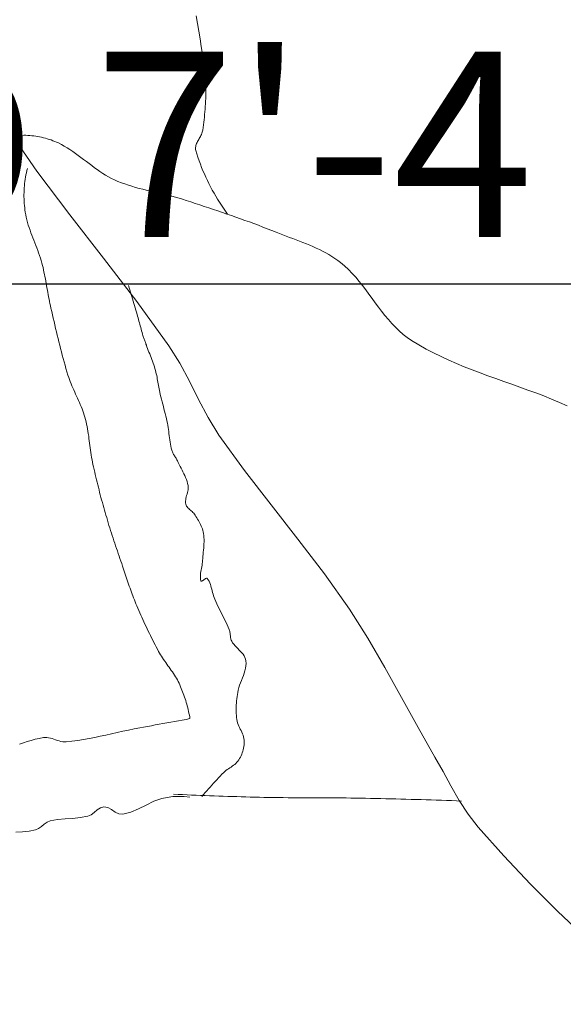
# Model space of a CAD drawing. Units: inches. Extents: x 2656 to 9931, y 1941 to 3068.
# Tile 17 of 46: x 2896 to 2914, y 2466 to 2498. Entities that reach past the tile are written whole.
import ezdxf

# ---------------------------------------------------------------- set-up
doc = ezdxf.new("R2010")
doc.units = ezdxf.units.IN
doc.layers.add('A-ANNO-DIMS', color=2, linetype='Continuous', lineweight=18)
doc.layers.add('A-FURN', color=8, linetype='Continuous', lineweight=13)
doc.styles.get("Standard").update_dxf_attribs({"font": 'arial.ttf'})
doc.dimstyles.new('ISO-25', dxfattribs={"dimtxt": 6, "dimasz": 2.5, "dimexe": 1.25, "dimexo": 0.625, "dimtad": 1, "dimdec": 0, "dimlunit": 3, "dimtxsty": 'Standard', "dimcen": 2.5, "dimadec": 0, "dimazin": 0, "dimtfac": 1, "dimtdec": 0, "dimtmove": 0, "dimatfit": 3, "dimfxl": 1, "dimarcsym": 0})

# ---------------------------------------------------------------- blocks, each defined once
blk = doc.blocks.new('BED-DOUBLE')
for p, q in [((24.852, 30.888), (24.895, 30.639)), ((24.895, 30.639), (24.937, 30.391)), ((24.937, 30.391), (24.978, 30.142)), ((24.978, 30.142), (25.017, 29.893)), ((25.017, 29.893), (25.054, 29.644)), ((25.054, 29.644), (25.087, 29.395)), ((25.087, 29.395), (25.118, 29.145)), ((25.118, 29.145), (25.146, 28.894)), ((25.146, 28.894), (25.153, 28.81)), ((25.153, 28.81), (25.159, 28.725)), ((25.159, 28.725), (25.164, 28.64)), ((25.164, 28.64), (25.166, 28.554)), ((25.166, 28.554), (25.168, 28.469)), ((25.168, 28.384), (25.166, 28.299)), ((25.168, 28.469), (25.168, 28.384)), ((25.155, 28.042), (25.149, 27.957)), ((25.16, 28.128), (25.155, 28.042)), ((25.163, 28.213), (25.16, 28.128)), ((25.166, 28.299), (25.163, 28.213)), ((25.127, 27.701), (25.118, 27.616)), ((25.135, 27.787), (25.127, 27.701)), ((25.142, 27.872), (25.135, 27.787)), ((25.149, 27.957), (25.142, 27.872)), ((25.098, 27.446), (25.088, 27.361)), ((25.108, 27.531), (25.098, 27.446)), ((25.118, 27.616), (25.108, 27.531)), ((18.699, 27.32), (19.702, 25.863)), ((25.04, 27.09), (25.026, 27.056)), ((25.052, 27.124), (25.04, 27.09)), ((25.061, 27.158), (25.052, 27.124)), ((25.067, 27.192), (25.061, 27.158)), ((25.078, 27.276), (25.067, 27.192)), ((25.088, 27.361), (25.078, 27.276)), ((19.217, 27.024), (19.153, 27.022)), ((19.28, 27.025), (19.217, 27.024)), ((19.344, 27.025), (19.28, 27.025)), ((19.408, 27.022), (19.344, 27.025)), ((19.472, 27.018), (19.408, 27.022)), ((19.535, 27.013), (19.472, 27.018)), ((19.599, 27.006), (19.535, 27.013)), ((19.663, 26.997), (19.599, 27.006)), ((19.726, 26.987), (19.663, 26.997)), ((19.789, 26.975), (19.726, 26.987)), ((19.852, 26.962), (19.789, 26.975)), ((19.915, 26.947), (19.852, 26.962)), ((19.977, 26.931), (19.915, 26.947)), ((20.039, 26.914), (19.977, 26.931)), ((20.1, 26.895), (20.039, 26.914)), ((20.16, 26.874), (20.1, 26.895)), ((20.22, 26.852), (20.16, 26.874)), ((20.28, 26.829), (20.22, 26.852)), ((20.338, 26.804), (20.28, 26.829)), ((20.396, 26.778), (20.338, 26.804)), ((20.493, 26.729), (20.396, 26.778)), ((24.869, 26.763), (24.856, 26.73)), ((24.884, 26.795), (24.869, 26.763)), ((24.901, 26.827), (24.884, 26.795)), ((24.919, 26.86), (24.901, 26.827)), ((24.937, 26.892), (24.919, 26.86)), ((24.956, 26.925), (24.937, 26.892)), ((24.975, 26.958), (24.956, 26.925)), ((24.993, 26.99), (24.975, 26.958)), ((25.01, 27.023), (24.993, 26.99)), ((25.026, 27.056), (25.01, 27.023)), ((20.588, 26.677), (20.493, 26.729)), ((20.681, 26.622), (20.588, 26.677)), ((20.773, 26.564), (20.681, 26.622)), ((20.863, 26.503), (20.773, 26.564)), ((20.952, 26.44), (20.863, 26.503)), ((21.04, 26.376), (20.952, 26.44)), ((24.833, 26.633), (24.832, 26.6)), ((24.832, 26.6), (24.835, 26.567)), ((24.838, 26.665), (24.833, 26.633)), ((24.835, 26.567), (24.842, 26.534)), ((24.845, 26.698), (24.838, 26.665)), ((24.842, 26.534), (24.876, 26.424)), ((24.856, 26.73), (24.845, 26.698)), ((24.876, 26.424), (24.912, 26.314)), ((21.128, 26.31), (21.04, 26.376)), ((21.215, 26.244), (21.128, 26.31)), ((21.302, 26.177), (21.215, 26.244)), ((21.389, 26.11), (21.302, 26.177)), ((21.476, 26.044), (21.389, 26.11)), ((24.912, 26.314), (24.949, 26.205)), ((24.949, 26.205), (24.989, 26.097)), ((19.362, 25.817), (19.348, 25.747)), ((19.377, 25.886), (19.362, 25.817)), ((19.394, 25.954), (19.377, 25.886)), ((19.702, 25.863), (20.765, 24.449)), ((21.563, 25.979), (21.476, 26.044)), ((21.652, 25.915), (21.563, 25.979)), ((21.741, 25.853), (21.652, 25.915)), ((21.832, 25.793), (21.741, 25.853)), ((21.924, 25.736), (21.832, 25.793)), ((24.989, 26.097), (25.031, 25.989)), ((25.031, 25.989), (25.074, 25.882)), ((25.074, 25.882), (25.12, 25.776)), ((19.314, 25.537), (19.306, 25.466)), ((19.324, 25.607), (19.314, 25.537)), ((19.335, 25.677), (19.324, 25.607)), ((19.348, 25.747), (19.335, 25.677)), ((22.018, 25.682), (21.924, 25.736)), ((22.114, 25.632), (22.018, 25.682)), ((22.211, 25.585), (22.114, 25.632)), ((22.322, 25.537), (22.211, 25.585)), ((22.434, 25.493), (22.322, 25.537)), ((22.547, 25.452), (22.434, 25.493)), ((25.12, 25.776), (25.167, 25.671)), ((25.167, 25.671), (25.216, 25.566)), ((25.216, 25.566), (25.267, 25.462)), ((19.286, 25.181), (19.285, 25.11)), ((19.289, 25.253), (19.286, 25.181)), ((19.293, 25.324), (19.289, 25.253)), ((19.299, 25.395), (19.293, 25.324)), ((19.306, 25.466), (19.299, 25.395)), ((22.661, 25.413), (22.547, 25.452)), ((22.775, 25.377), (22.661, 25.413)), ((22.891, 25.343), (22.775, 25.377)), ((23.007, 25.311), (22.891, 25.343)), ((23.124, 25.28), (23.007, 25.311)), ((23.241, 25.25), (23.124, 25.28)), ((23.359, 25.222), (23.241, 25.25)), ((23.476, 25.194), (23.359, 25.222)), ((23.594, 25.166), (23.476, 25.194)), ((23.712, 25.138), (23.594, 25.166)), ((25.267, 25.462), (25.32, 25.359)), ((25.32, 25.359), (25.374, 25.257)), ((25.374, 25.257), (25.431, 25.156)), ((25.431, 25.156), (25.489, 25.056)), ((19.285, 25.11), (19.285, 25.039)), ((19.285, 25.039), (19.287, 24.968)), ((19.287, 24.968), (19.289, 24.897)), ((19.289, 24.897), (19.294, 24.826)), ((23.83, 25.11), (23.712, 25.138)), ((23.948, 25.082), (23.83, 25.11)), ((24.065, 25.053), (23.948, 25.082)), ((24.182, 25.022), (24.065, 25.053)), ((24.299, 24.99), (24.182, 25.022)), ((24.414, 24.956), (24.299, 24.99)), ((24.53, 24.92), (24.414, 24.956)), ((24.676, 24.872), (24.53, 24.92)), ((24.823, 24.824), (24.676, 24.872)), ((25.489, 25.056), (25.548, 24.957)), ((25.548, 24.957), (25.61, 24.859)), ((25.61, 24.859), (25.673, 24.762)), ((19.294, 24.826), (19.3, 24.755)), ((19.3, 24.755), (19.307, 24.684)), ((19.307, 24.684), (19.315, 24.614)), ((19.315, 24.614), (19.325, 24.544)), ((19.325, 24.544), (19.34, 24.459)), ((24.97, 24.776), (24.823, 24.824)), ((25.117, 24.728), (24.97, 24.776)), ((25.263, 24.679), (25.117, 24.728)), ((25.41, 24.63), (25.263, 24.679)), ((25.556, 24.581), (25.41, 24.63)), ((25.702, 24.531), (25.556, 24.581)), ((25.673, 24.762), (25.737, 24.667)), ((25.848, 24.481), (25.702, 24.531)), ((25.737, 24.667), (25.804, 24.573)), ((25.804, 24.573), (25.871, 24.48)), ((19.34, 24.459), (19.358, 24.374)), ((19.358, 24.374), (19.378, 24.29)), ((19.378, 24.29), (19.401, 24.206)), ((19.401, 24.206), (19.425, 24.123)), ((20.765, 24.449), (21.855, 23.052)), ((25.994, 24.431), (25.848, 24.481)), ((26.14, 24.38), (25.994, 24.431)), ((26.285, 24.328), (26.14, 24.38)), ((26.431, 24.276), (26.285, 24.328)), ((26.576, 24.223), (26.431, 24.276)), ((26.72, 24.169), (26.576, 24.223)), ((19.425, 24.123), (19.452, 24.04)), ((19.452, 24.04), (19.48, 23.958)), ((19.48, 23.958), (19.509, 23.876)), ((19.509, 23.876), (19.54, 23.794)), ((26.865, 24.115), (26.72, 24.169)), ((27.009, 24.06), (26.865, 24.115)), ((27.153, 24.005), (27.009, 24.06)), ((27.297, 23.949), (27.153, 24.005)), ((27.44, 23.891), (27.297, 23.949)), ((27.548, 23.849), (27.44, 23.891)), ((19.54, 23.794), (19.571, 23.713)), ((19.571, 23.713), (19.603, 23.631)), ((19.603, 23.631), (19.635, 23.55)), ((27.656, 23.807), (27.548, 23.849)), ((27.764, 23.766), (27.656, 23.807)), ((27.873, 23.726), (27.764, 23.766)), ((27.982, 23.685), (27.873, 23.726)), ((28.092, 23.644), (27.982, 23.685)), ((28.201, 23.603), (28.092, 23.644)), ((28.309, 23.561), (28.201, 23.603)), ((28.418, 23.518), (28.309, 23.561)), ((19.635, 23.55), (19.666, 23.468)), ((19.666, 23.468), (19.698, 23.387)), ((19.698, 23.387), (19.729, 23.305)), ((19.729, 23.305), (19.758, 23.223)), ((28.525, 23.474), (28.418, 23.518)), ((28.632, 23.428), (28.525, 23.474)), ((28.738, 23.381), (28.632, 23.428)), ((28.842, 23.332), (28.738, 23.381)), ((28.945, 23.28), (28.842, 23.332)), ((29.047, 23.227), (28.945, 23.28)), ((19.758, 23.223), (19.787, 23.141)), ((19.787, 23.141), (19.814, 23.058)), ((19.814, 23.058), (19.84, 22.975)), ((19.84, 22.975), (19.864, 22.891)), ((21.855, 23.052), (22.936, 21.65)), ((29.147, 23.17), (29.047, 23.227)), ((29.245, 23.11), (29.147, 23.17)), ((29.341, 23.048), (29.245, 23.11)), ((29.434, 22.981), (29.341, 23.048)), ((29.526, 22.911), (29.434, 22.981)), ((19.864, 22.891), (19.882, 22.819)), ((19.882, 22.819), (19.9, 22.747)), ((19.9, 22.747), (19.917, 22.675)), ((19.917, 22.675), (19.932, 22.603)), ((19.932, 22.603), (19.947, 22.53)), ((29.656, 22.802), (29.526, 22.911)), ((29.78, 22.685), (29.656, 22.802)), ((29.898, 22.563), (29.78, 22.685)), ((19.947, 22.53), (19.962, 22.458)), ((19.962, 22.458), (19.976, 22.385)), ((19.976, 22.385), (19.99, 22.312)), ((19.99, 22.312), (20.003, 22.239)), ((30.013, 22.435), (29.898, 22.563)), ((30.123, 22.304), (30.013, 22.435)), ((30.231, 22.169), (30.123, 22.304)), ((20.003, 22.239), (20.016, 22.166)), ((20.016, 22.166), (20.029, 22.093)), ((20.029, 22.093), (20.042, 22.02)), ((20.042, 22.02), (20.055, 21.947)), ((22.664, 22.169), (22.686, 22.097)), ((22.686, 22.097), (22.708, 22.025)), ((22.708, 22.025), (22.73, 21.953)), ((30.336, 22.032), (30.231, 22.169)), ((30.44, 21.893), (30.336, 22.032)), ((20.055, 21.947), (20.068, 21.874)), ((20.068, 21.874), (20.082, 21.801)), ((20.082, 21.801), (20.095, 21.728)), ((20.095, 21.728), (20.11, 21.655)), ((20.11, 21.655), (20.125, 21.583)), ((22.73, 21.953), (22.752, 21.881)), ((22.752, 21.881), (22.774, 21.809)), ((22.774, 21.809), (22.796, 21.737)), ((22.796, 21.737), (22.817, 21.665)), ((22.817, 21.665), (22.839, 21.592)), ((22.936, 21.65), (23.974, 20.217)), ((30.543, 21.753), (30.44, 21.893)), ((30.646, 21.613), (30.543, 21.753)), ((20.125, 21.583), (20.14, 21.51)), ((20.14, 21.51), (20.157, 21.438)), ((20.157, 21.438), (20.182, 21.329)), ((20.182, 21.329), (20.207, 21.22)), ((22.839, 21.592), (22.86, 21.52)), ((22.86, 21.52), (22.881, 21.448)), ((22.881, 21.448), (22.902, 21.376)), ((22.902, 21.376), (22.923, 21.303)), ((30.749, 21.474), (30.646, 21.613)), ((30.853, 21.336), (30.749, 21.474)), ((30.96, 21.201), (30.853, 21.336)), ((20.207, 21.22), (20.232, 21.111)), ((20.232, 21.111), (20.258, 21.002)), ((22.923, 21.303), (22.944, 21.231)), ((22.944, 21.231), (22.959, 21.179)), ((22.959, 21.179), (22.974, 21.126)), ((22.974, 21.126), (22.988, 21.074)), ((22.988, 21.074), (23.003, 21.021)), ((23.003, 21.021), (23.017, 20.968)), ((31.069, 21.069), (30.96, 21.201)), ((31.181, 20.941), (31.069, 21.069)), ((20.258, 21.002), (20.283, 20.893)), ((20.283, 20.893), (20.308, 20.784)), ((20.308, 20.784), (20.334, 20.675)), ((23.017, 20.968), (23.03, 20.916)), ((23.03, 20.916), (23.044, 20.863)), ((23.044, 20.863), (23.059, 20.81)), ((23.059, 20.81), (23.073, 20.758)), ((23.073, 20.758), (23.087, 20.705)), ((23.087, 20.705), (23.102, 20.653)), ((31.298, 20.818), (31.181, 20.941)), ((31.419, 20.7), (31.298, 20.818)), ((31.546, 20.59), (31.419, 20.7)), ((20.334, 20.675), (20.36, 20.566)), ((20.36, 20.566), (20.386, 20.457)), ((20.386, 20.457), (20.412, 20.349)), ((23.102, 20.653), (23.117, 20.601)), ((23.117, 20.601), (23.133, 20.548)), ((23.133, 20.548), (23.142, 20.521)), ((23.142, 20.521), (23.151, 20.493)), ((23.151, 20.493), (23.16, 20.465)), ((23.16, 20.465), (23.17, 20.438)), ((23.17, 20.438), (23.18, 20.41)), ((23.18, 20.41), (23.19, 20.383)), ((23.19, 20.383), (23.2, 20.355)), ((31.68, 20.486), (31.546, 20.59)), ((31.82, 20.391), (31.68, 20.486)), ((32.053, 20.249), (31.82, 20.391)), ((20.412, 20.349), (20.439, 20.24)), ((20.439, 20.24), (20.467, 20.131)), ((20.467, 20.131), (20.494, 20.023)), ((23.2, 20.355), (23.211, 20.328)), ((23.211, 20.328), (23.221, 20.301)), ((23.221, 20.301), (23.231, 20.273)), ((23.231, 20.273), (23.242, 20.246)), ((23.242, 20.246), (23.252, 20.218)), ((23.252, 20.218), (23.262, 20.191)), ((23.262, 20.191), (23.283, 20.132)), ((23.283, 20.132), (23.305, 20.073)), ((23.305, 20.073), (23.328, 20.015)), ((23.974, 20.217), (24.323, 19.656)), ((32.29, 20.116), (32.053, 20.249)), ((32.531, 19.99), (32.29, 20.116)), ((20.494, 20.023), (20.523, 19.915)), ((20.523, 19.915), (20.552, 19.807)), ((20.552, 19.807), (20.581, 19.699)), ((23.328, 20.015), (23.35, 19.956)), ((23.35, 19.956), (23.373, 19.898)), ((23.373, 19.898), (23.396, 19.839)), ((23.396, 19.839), (23.418, 19.781)), ((23.418, 19.781), (23.44, 19.722)), ((32.775, 19.87), (32.531, 19.99)), ((33.022, 19.757), (32.775, 19.87)), ((33.272, 19.649), (33.022, 19.757)), ((20.581, 19.699), (20.612, 19.591)), ((20.612, 19.591), (20.643, 19.484)), ((20.643, 19.484), (20.675, 19.377)), ((23.44, 19.722), (23.461, 19.663)), ((23.461, 19.663), (23.482, 19.604)), ((23.482, 19.604), (23.502, 19.544)), ((23.502, 19.544), (23.521, 19.485)), ((23.521, 19.485), (23.538, 19.425)), ((23.538, 19.425), (23.552, 19.372)), ((24.323, 19.656), (24.634, 19.073)), ((33.525, 19.545), (33.272, 19.649)), ((33.779, 19.445), (33.525, 19.545)), ((34.035, 19.348), (33.779, 19.445)), ((20.675, 19.377), (20.708, 19.27)), ((20.708, 19.27), (20.73, 19.2)), ((20.73, 19.2), (20.755, 19.131)), ((20.755, 19.131), (20.781, 19.062)), ((23.552, 19.372), (23.565, 19.318)), ((23.565, 19.318), (23.577, 19.265)), ((23.577, 19.265), (23.587, 19.211)), ((23.587, 19.211), (23.597, 19.157)), ((23.597, 19.157), (23.607, 19.102)), ((23.607, 19.102), (23.616, 19.048)), ((34.292, 19.254), (34.035, 19.348)), ((34.55, 19.161), (34.292, 19.254)), ((34.809, 19.069), (34.55, 19.161)), ((20.781, 19.062), (20.808, 18.994)), ((20.808, 18.994), (20.836, 18.926)), ((20.836, 18.926), (20.865, 18.859)), ((20.865, 18.859), (20.895, 18.792)), ((20.895, 18.792), (20.925, 18.725)), ((23.616, 19.048), (23.625, 18.994)), ((23.625, 18.994), (23.634, 18.94)), ((23.634, 18.94), (23.643, 18.885)), ((23.643, 18.885), (23.653, 18.831)), ((23.653, 18.831), (23.664, 18.777)), ((24.634, 19.073), (24.932, 18.481)), ((35.068, 18.977), (34.809, 19.069)), ((35.326, 18.885), (35.068, 18.977)), ((35.584, 18.791), (35.326, 18.885)), ((35.841, 18.696), (35.584, 18.791)), ((20.925, 18.725), (20.956, 18.658)), ((20.956, 18.658), (20.987, 18.591)), ((20.987, 18.591), (21.017, 18.524)), ((21.017, 18.524), (21.048, 18.457)), ((23.664, 18.777), (23.675, 18.724)), ((23.675, 18.724), (23.693, 18.646)), ((23.693, 18.646), (23.712, 18.568)), ((23.712, 18.568), (23.732, 18.491)), ((23.732, 18.491), (23.751, 18.414)), ((24.932, 18.481), (25.243, 17.897)), ((36.097, 18.598), (35.841, 18.696)), ((36.351, 18.496), (36.097, 18.598)), ((36.603, 18.391), (36.351, 18.496)), ((21.048, 18.457), (21.078, 18.39)), ((21.078, 18.39), (21.107, 18.322)), ((21.107, 18.322), (21.135, 18.255)), ((21.135, 18.255), (21.162, 18.186)), ((21.162, 18.186), (21.188, 18.118)), ((23.751, 18.414), (23.771, 18.336)), ((23.771, 18.336), (23.792, 18.259)), ((23.792, 18.259), (23.812, 18.182)), ((23.812, 18.182), (23.832, 18.105)), ((36.853, 18.28), (36.603, 18.391)), ((21.188, 18.118), (21.213, 18.049)), ((21.213, 18.049), (21.235, 17.979)), ((21.235, 17.979), (21.256, 17.909)), ((21.256, 17.909), (21.276, 17.834)), ((21.276, 17.834), (21.294, 17.759)), ((23.832, 18.105), (23.851, 18.027)), ((23.851, 18.027), (23.87, 17.95)), ((23.87, 17.95), (23.889, 17.872)), ((23.889, 17.872), (23.907, 17.794)), ((25.243, 17.897), (25.59, 17.336)), ((21.294, 17.759), (21.311, 17.684)), ((21.311, 17.684), (21.326, 17.609)), ((21.326, 17.609), (21.34, 17.533)), ((21.34, 17.533), (21.353, 17.457)), ((23.907, 17.794), (23.923, 17.716)), ((23.923, 17.716), (23.936, 17.649)), ((23.936, 17.649), (23.948, 17.582)), ((23.948, 17.582), (23.958, 17.515)), ((23.958, 17.515), (23.967, 17.448)), ((21.353, 17.457), (21.365, 17.38)), ((21.365, 17.38), (21.377, 17.304)), ((21.377, 17.304), (21.387, 17.227)), ((21.387, 17.227), (21.398, 17.151)), ((23.967, 17.448), (23.975, 17.38)), ((23.975, 17.38), (23.984, 17.312)), ((23.984, 17.312), (23.992, 17.245)), ((23.992, 17.245), (24.001, 17.177)), ((25.59, 17.336), (26.414, 16.194)), ((21.398, 17.151), (21.408, 17.074)), ((21.408, 17.074), (21.418, 16.997)), ((21.418, 16.997), (21.428, 16.92)), ((21.428, 16.92), (21.439, 16.844)), ((24.001, 17.177), (24.011, 17.11)), ((24.011, 17.11), (24.022, 17.043)), ((24.022, 17.043), (24.034, 16.976)), ((24.034, 16.976), (24.049, 16.91)), ((24.049, 16.91), (24.065, 16.844)), ((21.439, 16.844), (21.45, 16.767)), ((21.45, 16.767), (21.461, 16.691)), ((21.461, 16.691), (21.473, 16.614)), ((21.473, 16.614), (21.487, 16.538)), ((24.065, 16.844), (24.073, 16.815)), ((24.073, 16.815), (24.084, 16.788)), ((24.084, 16.788), (24.096, 16.761)), ((24.096, 16.761), (24.109, 16.735)), ((24.109, 16.735), (24.124, 16.709)), ((24.124, 16.709), (24.139, 16.684)), ((24.139, 16.684), (24.155, 16.659)), ((24.155, 16.659), (24.171, 16.633)), ((24.171, 16.633), (24.187, 16.608)), ((24.187, 16.608), (24.203, 16.583)), ((24.203, 16.583), (24.218, 16.557)), ((24.218, 16.557), (24.232, 16.531)), ((21.487, 16.538), (21.501, 16.462)), ((21.501, 16.462), (21.516, 16.386)), ((21.516, 16.386), (21.534, 16.304)), ((21.534, 16.304), (21.553, 16.221)), ((24.232, 16.531), (24.245, 16.504)), ((24.245, 16.504), (24.274, 16.444)), ((24.274, 16.444), (24.304, 16.384)), ((24.304, 16.384), (24.335, 16.323)), ((24.335, 16.323), (24.366, 16.264)), ((24.366, 16.264), (24.397, 16.203)), ((21.553, 16.221), (21.571, 16.139)), ((21.571, 16.139), (21.59, 16.056)), ((21.59, 16.056), (21.609, 15.974)), ((21.609, 15.974), (21.629, 15.892)), ((24.397, 16.203), (24.427, 16.143)), ((24.427, 16.143), (24.457, 16.083)), ((24.457, 16.083), (24.485, 16.022)), ((24.485, 16.022), (24.512, 15.96)), ((24.512, 15.96), (24.536, 15.898)), ((26.414, 16.194), (27.275, 15.078)), ((21.629, 15.892), (21.649, 15.809)), ((21.649, 15.809), (21.669, 15.727)), ((21.669, 15.727), (21.69, 15.645)), ((21.69, 15.645), (21.711, 15.563)), ((24.536, 15.898), (24.558, 15.835)), ((24.558, 15.835), (24.576, 15.771)), ((24.576, 15.771), (24.591, 15.705)), ((24.591, 15.705), (24.596, 15.659)), ((24.596, 15.613), (24.591, 15.567)), ((24.596, 15.659), (24.596, 15.613)), ((21.711, 15.563), (21.732, 15.481)), ((21.732, 15.481), (21.753, 15.4)), ((21.753, 15.4), (21.775, 15.318)), ((21.775, 15.318), (21.797, 15.236)), ((24.522, 15.287), (24.515, 15.24)), ((24.533, 15.333), (24.522, 15.287)), ((24.545, 15.38), (24.533, 15.333)), ((24.559, 15.427), (24.545, 15.38)), ((24.571, 15.473), (24.559, 15.427)), ((24.583, 15.52), (24.571, 15.473)), ((24.591, 15.567), (24.583, 15.52)), ((21.797, 15.236), (21.819, 15.154)), ((21.819, 15.154), (21.842, 15.073)), ((21.842, 15.073), (21.865, 14.991)), ((21.865, 14.991), (21.888, 14.91)), ((24.515, 15.24), (24.511, 15.194)), ((24.511, 15.194), (24.512, 15.148)), ((24.512, 15.148), (24.519, 15.103)), ((24.519, 15.103), (24.53, 15.069)), ((24.53, 15.069), (24.546, 15.038)), ((24.546, 15.038), (24.565, 15.009)), ((24.565, 15.009), (24.588, 14.982)), ((24.588, 14.982), (24.613, 14.956)), ((27.275, 15.078), (28.146, 13.969)), ((21.888, 14.91), (21.911, 14.829)), ((21.911, 14.829), (21.934, 14.748)), ((21.934, 14.748), (21.959, 14.664)), ((21.959, 14.664), (21.984, 14.581)), ((24.613, 14.956), (24.639, 14.931)), ((24.639, 14.931), (24.667, 14.907)), ((24.667, 14.907), (24.696, 14.882)), ((24.696, 14.882), (24.724, 14.858)), ((24.724, 14.858), (24.751, 14.833)), ((24.751, 14.833), (24.777, 14.806)), ((24.777, 14.806), (24.8, 14.779)), ((24.8, 14.779), (24.82, 14.749)), ((24.82, 14.749), (24.846, 14.706)), ((24.846, 14.706), (24.873, 14.662)), ((24.873, 14.662), (24.899, 14.619)), ((21.984, 14.581), (22.009, 14.498)), ((22.009, 14.498), (22.034, 14.415)), ((22.034, 14.415), (22.06, 14.332)), ((22.06, 14.332), (22.086, 14.249)), ((24.899, 14.619), (24.924, 14.575)), ((24.924, 14.575), (24.949, 14.53)), ((24.949, 14.53), (24.974, 14.485)), ((24.974, 14.485), (24.996, 14.44)), ((24.996, 14.44), (25.018, 14.394)), ((25.018, 14.394), (25.037, 14.347)), ((25.037, 14.347), (25.055, 14.3)), ((22.086, 14.249), (22.113, 14.166)), ((22.113, 14.166), (22.14, 14.083)), ((22.14, 14.083), (22.167, 14.001)), ((25.055, 14.3), (25.07, 14.252)), ((25.07, 14.252), (25.083, 14.204)), ((25.083, 14.204), (25.092, 14.155)), ((25.092, 14.155), (25.101, 14.088)), ((25.101, 14.088), (25.107, 14.021)), ((25.107, 14.021), (25.11, 13.954)), ((22.167, 14.001), (22.194, 13.918)), ((22.194, 13.918), (22.221, 13.835)), ((22.221, 13.835), (22.249, 13.753)), ((22.249, 13.753), (22.277, 13.671)), ((25.103, 13.751), (25.098, 13.684)), ((25.107, 13.819), (25.103, 13.751)), ((25.11, 13.886), (25.107, 13.819)), ((25.11, 13.954), (25.11, 13.886)), ((28.146, 13.969), (29.001, 12.85)), ((22.277, 13.671), (22.304, 13.588)), ((22.304, 13.588), (22.332, 13.506)), ((22.332, 13.506), (22.36, 13.424)), ((22.36, 13.424), (22.388, 13.341)), ((25.072, 13.413), (25.066, 13.345)), ((25.078, 13.48), (25.072, 13.413)), ((25.085, 13.548), (25.078, 13.48)), ((25.092, 13.616), (25.085, 13.548)), ((25.098, 13.684), (25.092, 13.616)), ((22.388, 13.341), (22.417, 13.259)), ((22.417, 13.259), (22.445, 13.177)), ((22.445, 13.177), (22.473, 13.094)), ((22.473, 13.094), (22.495, 13.03)), ((25.034, 13.075), (25.024, 13.024)), ((25.043, 13.126), (25.034, 13.075)), ((25.051, 13.177), (25.043, 13.126)), ((25.058, 13.227), (25.051, 13.177)), ((25.062, 13.278), (25.058, 13.227)), ((25.066, 13.345), (25.062, 13.278)), ((22.495, 13.03), (22.516, 12.966)), ((22.516, 12.966), (22.538, 12.901)), ((22.538, 12.901), (22.56, 12.837)), ((22.56, 12.837), (22.581, 12.773)), ((22.581, 12.773), (22.603, 12.708)), ((24.994, 12.822), (24.992, 12.772)), ((24.992, 12.772), (24.994, 12.722)), ((24.999, 12.872), (24.994, 12.822)), ((25.006, 12.923), (24.999, 12.872)), ((25.015, 12.973), (25.006, 12.923)), ((25.024, 13.024), (25.015, 12.973)), ((29.001, 12.85), (29.816, 11.701)), ((22.603, 12.708), (22.625, 12.644)), ((22.625, 12.644), (22.647, 12.58)), ((22.647, 12.58), (22.669, 12.516)), ((22.669, 12.516), (22.692, 12.451)), ((22.692, 12.451), (22.714, 12.387)), ((24.994, 12.722), (24.999, 12.673)), ((24.999, 12.673), (25.009, 12.624)), ((25.009, 12.624), (25.016, 12.612)), ((25.016, 12.612), (25.026, 12.609)), ((25.026, 12.609), (25.039, 12.612)), ((25.039, 12.612), (25.055, 12.621)), ((25.055, 12.621), (25.073, 12.633)), ((25.073, 12.633), (25.092, 12.648)), ((25.092, 12.648), (25.112, 12.664)), ((25.112, 12.664), (25.132, 12.679)), ((25.132, 12.679), (25.152, 12.693)), ((25.152, 12.693), (25.17, 12.702)), ((25.17, 12.702), (25.187, 12.708)), ((25.187, 12.708), (25.202, 12.706)), ((25.202, 12.706), (25.214, 12.697)), ((25.214, 12.697), (25.244, 12.653)), ((25.244, 12.653), (25.27, 12.606)), ((25.27, 12.606), (25.292, 12.557)), ((25.292, 12.557), (25.312, 12.507)), ((25.312, 12.507), (25.329, 12.455)), ((25.329, 12.455), (25.344, 12.402)), ((22.714, 12.387), (22.737, 12.324)), ((22.737, 12.324), (22.76, 12.26)), ((22.76, 12.26), (22.784, 12.196)), ((22.784, 12.196), (22.807, 12.132)), ((22.807, 12.132), (22.832, 12.069)), ((25.344, 12.402), (25.358, 12.349)), ((25.358, 12.349), (25.372, 12.295)), ((25.372, 12.295), (25.386, 12.242)), ((25.386, 12.242), (25.4, 12.188)), ((25.4, 12.188), (25.416, 12.136)), ((25.416, 12.136), (25.433, 12.084)), ((22.832, 12.069), (22.856, 12.006)), ((22.856, 12.006), (22.881, 11.943)), ((22.881, 11.943), (22.907, 11.88)), ((22.907, 11.88), (22.933, 11.817)), ((22.933, 11.817), (22.965, 11.742)), ((25.433, 12.084), (25.453, 12.033)), ((25.453, 12.033), (25.487, 11.956)), ((25.487, 11.956), (25.522, 11.88)), ((25.522, 11.88), (25.559, 11.805)), ((25.559, 11.805), (25.596, 11.729)), ((22.965, 11.742), (22.998, 11.667)), ((22.998, 11.667), (23.03, 11.592)), ((23.03, 11.592), (23.063, 11.517)), ((23.063, 11.517), (23.097, 11.442)), ((25.596, 11.729), (25.634, 11.654)), ((25.634, 11.654), (25.672, 11.579)), ((25.672, 11.579), (25.71, 11.505)), ((25.71, 11.505), (25.748, 11.43)), ((29.816, 11.701), (30.407, 10.77)), ((23.097, 11.442), (23.13, 11.367)), ((23.13, 11.367), (23.164, 11.293)), ((23.164, 11.293), (23.198, 11.218)), ((23.198, 11.218), (23.233, 11.144)), ((23.233, 11.144), (23.268, 11.07)), ((25.748, 11.43), (25.786, 11.354)), ((25.786, 11.354), (25.822, 11.279)), ((25.822, 11.279), (25.857, 11.203)), ((25.857, 11.203), (25.891, 11.126)), ((23.268, 11.07), (23.303, 10.996)), ((23.303, 10.996), (23.339, 10.922)), ((23.339, 10.922), (23.375, 10.849)), ((23.375, 10.849), (23.412, 10.775)), ((25.891, 11.126), (25.924, 11.048)), ((25.924, 11.048), (25.933, 11.021)), ((25.933, 11.021), (25.941, 10.992)), ((25.941, 10.992), (25.946, 10.963)), ((25.946, 10.963), (25.951, 10.933)), ((25.951, 10.933), (25.954, 10.903)), ((25.954, 10.903), (25.957, 10.873)), ((25.957, 10.873), (25.959, 10.843)), ((25.959, 10.843), (25.963, 10.813)), ((23.412, 10.775), (23.449, 10.702)), ((23.449, 10.702), (23.486, 10.629)), ((23.486, 10.629), (23.524, 10.557)), ((23.524, 10.557), (23.562, 10.484)), ((25.963, 10.813), (25.967, 10.784)), ((25.967, 10.784), (25.972, 10.755)), ((25.972, 10.755), (25.98, 10.727)), ((25.98, 10.727), (25.989, 10.699)), ((25.989, 10.699), (26.002, 10.672)), ((26.002, 10.672), (26.033, 10.62)), ((26.033, 10.62), (26.07, 10.57)), ((26.07, 10.57), (26.111, 10.522)), ((26.111, 10.522), (26.155, 10.476)), ((30.407, 10.77), (30.961, 9.816)), ((23.562, 10.484), (23.6, 10.412)), ((23.6, 10.412), (23.639, 10.34)), ((23.639, 10.34), (23.669, 10.287)), ((23.669, 10.287), (23.7, 10.234)), ((23.7, 10.234), (23.733, 10.182)), ((26.155, 10.476), (26.2, 10.43)), ((26.2, 10.43), (26.245, 10.385)), ((26.245, 10.385), (26.289, 10.34)), ((26.289, 10.34), (26.332, 10.293)), ((26.332, 10.293), (26.37, 10.246)), ((26.37, 10.246), (26.404, 10.196)), ((26.404, 10.196), (26.432, 10.144)), ((23.733, 10.182), (23.766, 10.131)), ((23.766, 10.131), (23.8, 10.08)), ((23.8, 10.08), (23.835, 10.029)), ((23.835, 10.029), (23.871, 9.979)), ((23.871, 9.979), (23.906, 9.928)), ((23.906, 9.928), (23.942, 9.878)), ((23.942, 9.878), (23.978, 9.828)), ((26.432, 10.144), (26.452, 10.089)), ((26.464, 9.871), (26.451, 9.793)), ((26.452, 10.089), (26.464, 10.031)), ((26.464, 10.031), (26.468, 9.951)), ((26.468, 9.951), (26.464, 9.871)), ((23.978, 9.828), (24.014, 9.778)), ((24.014, 9.778), (24.049, 9.728)), ((24.049, 9.728), (24.084, 9.677)), ((24.084, 9.677), (24.118, 9.627)), ((24.118, 9.627), (24.151, 9.575)), ((24.151, 9.575), (24.184, 9.523)), ((26.381, 9.559), (26.351, 9.481)), ((26.408, 9.637), (26.381, 9.559)), ((26.432, 9.714), (26.408, 9.637)), ((26.451, 9.793), (26.432, 9.714)), ((30.961, 9.816), (31.497, 8.85)), ((24.184, 9.523), (24.215, 9.471)), ((24.215, 9.471), (24.245, 9.417)), ((24.245, 9.417), (24.273, 9.363)), ((24.273, 9.363), (24.3, 9.308)), ((24.3, 9.308), (24.325, 9.254)), ((24.325, 9.254), (24.349, 9.199)), ((26.26, 9.248), (26.234, 9.17)), ((26.289, 9.326), (26.26, 9.248)), ((26.32, 9.404), (26.289, 9.326)), ((26.351, 9.481), (26.32, 9.404)), ((24.349, 9.199), (24.372, 9.144)), ((24.372, 9.144), (24.395, 9.088)), ((24.395, 9.088), (24.417, 9.033)), ((24.417, 9.033), (24.438, 8.977)), ((24.438, 8.977), (24.459, 8.92)), ((24.459, 8.92), (24.479, 8.863)), ((26.187, 8.944), (26.177, 8.877)), ((26.197, 9.011), (26.187, 8.944)), ((26.212, 9.091), (26.197, 9.011)), ((26.234, 9.17), (26.212, 9.091)), ((24.479, 8.863), (24.497, 8.806)), ((24.497, 8.806), (24.516, 8.749)), ((24.516, 8.749), (24.533, 8.692)), ((24.533, 8.692), (24.55, 8.634)), ((24.55, 8.634), (24.566, 8.576)), ((26.152, 8.607), (26.148, 8.539)), ((26.156, 8.674), (26.152, 8.607)), ((26.162, 8.742), (26.156, 8.674)), ((26.169, 8.81), (26.162, 8.742)), ((26.177, 8.877), (26.169, 8.81)), ((31.497, 8.85), (32.03, 7.883)), ((24.566, 8.576), (24.581, 8.518)), ((24.581, 8.518), (24.595, 8.46)), ((24.595, 8.46), (24.608, 8.401)), ((24.608, 8.401), (24.621, 8.342)), ((24.621, 8.342), (24.633, 8.284)), ((24.633, 8.284), (24.644, 8.225)), ((26.148, 8.539), (26.147, 8.471)), ((26.147, 8.471), (26.147, 8.403)), ((26.147, 8.403), (26.149, 8.336)), ((26.149, 8.336), (26.153, 8.268)), ((23.529, 7.962), (23.404, 7.939)), ((23.654, 7.985), (23.529, 7.962)), ((23.779, 8.008), (23.654, 7.985)), ((23.904, 8.031), (23.779, 8.008)), ((24.029, 8.053), (23.904, 8.031)), ((24.154, 8.076), (24.029, 8.053)), ((24.279, 8.099), (24.154, 8.076)), ((24.404, 8.121), (24.279, 8.099)), ((24.529, 8.144), (24.404, 8.121)), ((24.654, 8.166), (24.529, 8.144)), ((24.644, 8.225), (24.654, 8.166)), ((26.153, 8.268), (26.158, 8.201)), ((26.158, 8.201), (26.166, 8.134)), ((26.166, 8.134), (26.177, 8.081)), ((26.177, 8.081), (26.191, 8.029)), ((26.191, 8.029), (26.21, 7.978)), ((26.21, 7.978), (26.232, 7.927)), ((22.118, 7.677), (21.936, 7.637)), ((22.3, 7.717), (22.118, 7.677)), ((22.482, 7.757), (22.3, 7.717)), ((22.664, 7.796), (22.482, 7.757)), ((22.847, 7.833), (22.664, 7.796)), ((23.029, 7.869), (22.847, 7.833)), ((23.154, 7.892), (23.029, 7.869)), ((23.279, 7.915), (23.154, 7.892)), ((23.404, 7.939), (23.279, 7.915)), ((26.232, 7.927), (26.256, 7.877)), ((26.256, 7.877), (26.281, 7.828)), ((26.281, 7.828), (26.306, 7.778)), ((26.306, 7.778), (26.33, 7.728)), ((26.33, 7.728), (26.353, 7.678)), ((26.353, 7.678), (26.373, 7.627)), ((32.03, 7.883), (32.577, 6.925)), ((19.264, 7.386), (19.137, 7.343)), ((19.392, 7.427), (19.264, 7.386)), ((19.52, 7.464), (19.392, 7.427)), ((19.649, 7.498), (19.52, 7.464)), ((19.779, 7.528), (19.649, 7.498)), ((19.911, 7.552), (19.779, 7.528)), ((19.968, 7.558), (19.911, 7.552)), ((20.025, 7.556), (19.968, 7.558)), ((20.082, 7.548), (20.025, 7.556)), ((20.139, 7.535), (20.082, 7.548)), ((20.196, 7.519), (20.139, 7.535)), ((20.252, 7.5), (20.196, 7.519)), ((20.309, 7.48), (20.252, 7.5)), ((20.366, 7.461), (20.309, 7.48)), ((20.423, 7.444), (20.366, 7.461)), ((20.48, 7.429), (20.423, 7.444)), ((20.538, 7.419), (20.48, 7.429)), ((20.595, 7.414), (20.538, 7.419)), ((20.653, 7.416), (20.595, 7.414)), ((20.837, 7.437), (20.653, 7.416)), ((21.022, 7.463), (20.837, 7.437)), ((21.205, 7.492), (21.022, 7.463)), ((21.388, 7.525), (21.205, 7.492)), ((21.571, 7.56), (21.388, 7.525)), ((21.754, 7.598), (21.571, 7.56)), ((21.936, 7.637), (21.754, 7.598)), ((26.373, 7.627), (26.389, 7.576)), ((26.389, 7.576), (26.4, 7.524)), ((26.4, 7.524), (26.406, 7.47)), ((26.406, 7.367), (26.402, 7.316)), ((26.406, 7.47), (26.407, 7.419)), ((26.407, 7.419), (26.406, 7.367)), ((26.326, 7.014), (26.306, 6.966)), ((26.344, 7.063), (26.326, 7.014)), ((26.36, 7.112), (26.344, 7.063)), ((26.374, 7.163), (26.36, 7.112)), ((26.386, 7.213), (26.374, 7.163)), ((26.395, 7.265), (26.386, 7.213)), ((26.402, 7.316), (26.395, 7.265)), ((26.102, 6.688), (26.063, 6.658)), ((26.139, 6.72), (26.102, 6.688)), ((26.173, 6.754), (26.139, 6.72)), ((26.205, 6.791), (26.173, 6.754)), ((26.233, 6.83), (26.205, 6.791)), ((26.259, 6.874), (26.233, 6.83)), ((26.283, 6.919), (26.259, 6.874)), ((26.306, 6.966), (26.283, 6.919)), ((32.577, 6.925), (32.84, 6.459)), ((25.744, 6.423), (25.687, 6.366)), ((25.78, 6.456), (25.744, 6.423)), ((25.818, 6.488), (25.78, 6.456)), ((25.858, 6.517), (25.818, 6.488)), ((25.899, 6.546), (25.858, 6.517)), ((25.94, 6.574), (25.899, 6.546)), ((25.982, 6.601), (25.94, 6.574)), ((26.023, 6.63), (25.982, 6.601)), ((26.063, 6.658), (26.023, 6.63)), ((32.84, 6.459), (33.095, 5.989)), ((25.41, 6.076), (25.356, 6.016)), ((25.465, 6.135), (25.41, 6.076)), ((25.52, 6.193), (25.465, 6.135)), ((25.575, 6.251), (25.52, 6.193)), ((25.631, 6.309), (25.575, 6.251)), ((25.687, 6.366), (25.631, 6.309)), ((25.144, 5.774), (25.093, 5.712)), ((25.197, 5.835), (25.144, 5.774)), ((25.249, 5.896), (25.197, 5.835)), ((25.302, 5.956), (25.249, 5.896)), ((25.356, 6.016), (25.302, 5.956)), ((33.095, 5.989), (33.36, 5.524)), ((23.481, 5.494), (23.234, 5.374)), ((23.738, 5.584), (23.481, 5.494)), ((23.917, 5.622), (23.738, 5.584)), ((24.099, 5.644), (23.917, 5.622)), ((24.282, 5.652), (24.099, 5.644)), ((24.267, 5.715), (24.121, 5.722)), ((24.413, 5.709), (24.267, 5.715)), ((24.466, 5.645), (24.282, 5.652)), ((24.559, 5.702), (24.413, 5.709)), ((24.647, 5.623), (24.466, 5.645)), ((24.705, 5.696), (24.559, 5.702)), ((24.851, 5.69), (24.705, 5.696)), ((24.997, 5.684), (24.851, 5.69)), ((25.143, 5.678), (24.997, 5.684)), ((25.093, 5.712), (25.042, 5.65)), ((25.29, 5.673), (25.143, 5.678)), ((25.436, 5.667), (25.29, 5.673)), ((25.582, 5.662), (25.436, 5.667)), ((25.728, 5.657), (25.582, 5.662)), ((25.874, 5.653), (25.728, 5.657)), ((26.02, 5.648), (25.874, 5.653)), ((26.166, 5.644), (26.02, 5.648)), ((26.313, 5.64), (26.166, 5.644)), ((26.459, 5.636), (26.313, 5.64)), ((26.605, 5.632), (26.459, 5.636)), ((26.751, 5.628), (26.605, 5.632)), ((26.897, 5.625), (26.751, 5.628)), ((27.044, 5.622), (26.897, 5.625)), ((27.2, 5.619), (27.044, 5.622)), ((27.356, 5.616), (27.2, 5.619)), ((27.513, 5.614), (27.356, 5.616)), ((27.669, 5.612), (27.513, 5.614)), ((27.825, 5.611), (27.669, 5.612)), ((27.982, 5.61), (27.825, 5.611)), ((28.138, 5.609), (27.982, 5.61)), ((28.294, 5.608), (28.138, 5.609)), ((28.451, 5.608), (28.294, 5.608)), ((28.607, 5.607), (28.451, 5.608)), ((28.763, 5.607), (28.607, 5.607)), ((28.92, 5.606), (28.763, 5.607)), ((29.076, 5.606), (28.92, 5.606)), ((29.232, 5.605), (29.076, 5.606)), ((29.389, 5.604), (29.232, 5.605)), ((29.545, 5.603), (29.389, 5.604)), ((29.702, 5.601), (29.545, 5.603)), ((29.858, 5.6), (29.702, 5.601)), ((30.014, 5.597), (29.858, 5.6)), ((30.171, 5.595), (30.014, 5.597)), ((30.334, 5.592), (30.171, 5.595)), ((30.497, 5.588), (30.334, 5.592)), ((30.661, 5.585), (30.497, 5.588)), ((30.824, 5.581), (30.661, 5.585)), ((30.987, 5.578), (30.824, 5.581)), ((31.151, 5.574), (30.987, 5.578)), ((31.314, 5.57), (31.151, 5.574)), ((31.477, 5.565), (31.314, 5.57)), ((31.64, 5.561), (31.477, 5.565)), ((31.804, 5.556), (31.64, 5.561)), ((31.967, 5.552), (31.804, 5.556)), ((32.13, 5.547), (31.967, 5.552)), ((32.294, 5.542), (32.13, 5.547)), ((32.457, 5.537), (32.294, 5.542)), ((32.62, 5.531), (32.457, 5.537)), ((32.784, 5.526), (32.62, 5.531)), ((32.947, 5.52), (32.784, 5.526)), ((33.11, 5.515), (32.947, 5.52)), ((33.273, 5.509), (33.11, 5.515)), ((33.437, 5.503), (33.273, 5.509)), ((33.36, 5.524), (33.647, 5.076)), ((21.558, 5.137), (21.457, 5.061)), ((21.656, 5.218), (21.558, 5.137)), ((21.758, 5.284), (21.656, 5.218)), ((21.872, 5.315), (21.758, 5.284)), ((21.998, 5.292), (21.872, 5.315)), ((22.118, 5.226), (21.998, 5.292)), ((22.235, 5.148), (22.118, 5.226)), ((22.354, 5.087), (22.235, 5.148)), ((22.74, 5.14), (22.479, 5.073)), ((22.989, 5.248), (22.74, 5.14)), ((23.234, 5.374), (22.989, 5.248)), ((20.03, 4.818), (19.938, 4.753)), ((20.131, 4.861), (20.03, 4.818)), ((20.371, 4.906), (20.131, 4.861)), ((20.616, 4.928), (20.371, 4.906)), ((20.862, 4.943), (20.616, 4.928)), ((21.107, 4.965), (20.862, 4.943)), ((21.347, 5.011), (21.107, 4.965)), ((21.457, 5.061), (21.347, 5.011)), ((22.479, 5.073), (22.354, 5.087)), ((33.647, 5.076), (33.973, 4.657)), ((19.236, 4.507), (19.022, 4.492)), ((19.448, 4.533), (19.236, 4.507)), ((19.657, 4.574), (19.448, 4.533)), ((19.758, 4.617), (19.657, 4.574)), ((19.85, 4.681), (19.758, 4.617)), ((19.938, 4.753), (19.85, 4.681)), ((33.973, 4.657), (34.806, 3.726)), ((34.806, 3.726), (35.666, 2.819)), ((35.666, 2.819), (36.55, 1.936)), ((36.55, 1.936), (37.459, 1.078))]:
    blk.add_line(p, q)
blk = doc.blocks.new('*D31')
at = {"layer": 'A-ANNO-DIMS', "color": 0, "lineweight": -2, "transparency": 16777216}
for p, q in [((2753.358, 2502.145), (2753.358, 2488.227)), ((2841.982, 2502.145), (2841.982, 2488.227)), ((2755.858, 2489.477), (2839.482, 2489.477)), ((2841.982, 2489.477), (2952.348, 2489.477))]:
    blk.add_line(p, q, dxfattribs=at)
at = {"layer": 'A-ANNO-DIMS', "color": 0, "transparency": 16777216}
for points in [[(2755.858, 2489.893), (2755.858, 2489.06), (2753.358, 2489.477)], [(2839.482, 2489.893), (2839.482, 2489.06), (2841.982, 2489.477)]]:
    blk.add_solid(points, dxfattribs=at)
at = {"layer": 'Defpoints', "color": 0, "transparency": 16777216}
for p in [(2753.358, 2502.77), (2841.982, 2502.77), (2841.982, 2489.477)]:
    blk.add_point(p, dxfattribs=at)
at = {"layer": 'A-ANNO-DIMS', "color": 0, "transparency": 16777216, "insert": (2898.415, 2493.206), "char_height": 6, "attachment_point": 5}
blk.add_mtext('DOUBLE BED 7\'-4 1/2" TYP.', dxfattribs=at)
blk = doc.blocks.new('*D102')
at = {"layer": 'A-ANNO-DIMS', "color": 0, "lineweight": -2, "transparency": 16777216}
for p, q in [((2998.157, 2604.975), (2998.157, 2009.273)), ((2872.157, 2564.712), (2872.157, 2009.273)), ((2874.657, 2010.523), (2995.657, 2010.523))]:
    blk.add_line(p, q, dxfattribs=at)
at = {"layer": 'A-ANNO-DIMS', "color": 0, "transparency": 16777216}
for points in [[(2874.657, 2010.939), (2874.657, 2010.106), (2872.157, 2010.523)], [(2995.657, 2010.939), (2995.657, 2010.106), (2998.157, 2010.523)]]:
    blk.add_solid(points, dxfattribs=at)
at = {"layer": 'Defpoints', "color": 0, "transparency": 16777216}
for p in [(2998.157, 2605.6), (2872.157, 2565.337), (2998.157, 2010.523)]:
    blk.add_point(p, dxfattribs=at)
at = {"layer": 'A-ANNO-DIMS', "color": 0, "transparency": 16777216, "insert": (2935.157, 2014.211), "char_height": 6, "attachment_point": 5}
blk.add_mtext('10\'-6"', dxfattribs=at)
blk = doc.blocks.new('*D130')
at = {"layer": 'A-ANNO-DIMS', "color": 0, "lineweight": -2, "transparency": 16777216}
for p, q in [((2877.282, 2538.52), (3061.007, 2538.52)), ((3059.757, 2536.02), (3059.757, 2525.316)), ((2902.165, 2522.816), (3061.007, 2522.816)), ((3059.757, 2522.816), (3059.757, 2489.7))]:
    blk.add_line(p, q, dxfattribs=at)
at = {"layer": 'A-ANNO-DIMS', "color": 0, "transparency": 16777216}
for points in [[(3059.341, 2536.02), (3060.174, 2536.02), (3059.757, 2538.52)], [(3059.341, 2525.316), (3060.174, 2525.316), (3059.757, 2522.816)]]:
    blk.add_solid(points, dxfattribs=at)
at = {"layer": 'Defpoints', "color": 0, "transparency": 16777216}
for p in [(2876.657, 2538.52), (2901.54, 2522.816), (3059.757, 2522.816)]:
    blk.add_point(p, dxfattribs=at)
at = {"layer": 'A-ANNO-DIMS', "color": 0, "transparency": 16777216, "insert": (3056.028, 2505.008), "char_height": 6, "attachment_point": 5, "rotation": 90}
blk.add_mtext('1\'-3 1/2"', dxfattribs=at)

msp = doc.modelspace()

# ---------------------------------------------------------------- block references
at = {"layer": 'A-FURN'}
msp.add_blockref('BED-DOUBLE', (2877.353, 2467.251), dxfattribs=at)

# ---------------------------------------------------------------- dimensions: what is measured, and where the dimension line sits
at = {"layer": 'A-ANNO-DIMS'}
dim = msp.add_linear_dim(base=(2998.157, 2010.523), p1=(2872.157, 2565.337), p2=(2998.157, 2605.6), dimstyle='ISO-25', override={"dimdec": 1, "dimlfac": 1, "dimrnd": 0, "dimzin": 1, "dimdsep": 46, "dimlunit": 4, "dimfrac": 2}, dxfattribs=at)
dim.commit()
dim.dimension.update_dxf_attribs({"geometry": '*D102', "text_midpoint": (2935.157, 2014.211)})
dim = msp.add_linear_dim(base=(3059.757, 2522.816), p1=(2876.657, 2538.52), p2=(2901.54, 2522.816), angle=90, dimstyle='ISO-25', override={"dimdec": 1, "dimlfac": 1, "dimrnd": 0, "dimzin": 1, "dimdsep": 46, "dimlunit": 4, "dimfrac": 2}, dxfattribs=at)
dim.commit()
dim.dimension.update_dxf_attribs({"geometry": '*D130', "text_midpoint": (3056.028, 2505.008)})
dim = msp.add_linear_dim(base=(2841.982, 2489.477), p1=(2753.358, 2502.77), p2=(2841.982, 2502.77), text='DOUBLE BED <> TYP.', dimstyle='ISO-25', override={"dimdec": 1, "dimlfac": 1, "dimrnd": 0, "dimzin": 1, "dimdsep": 46, "dimlunit": 4, "dimfrac": 2}, dxfattribs=at)
dim.commit()
dim.dimension.update_dxf_attribs({"geometry": '*D31', "text_midpoint": (2898.415, 2493.206)})

doc.saveas('drawing.dxf')
